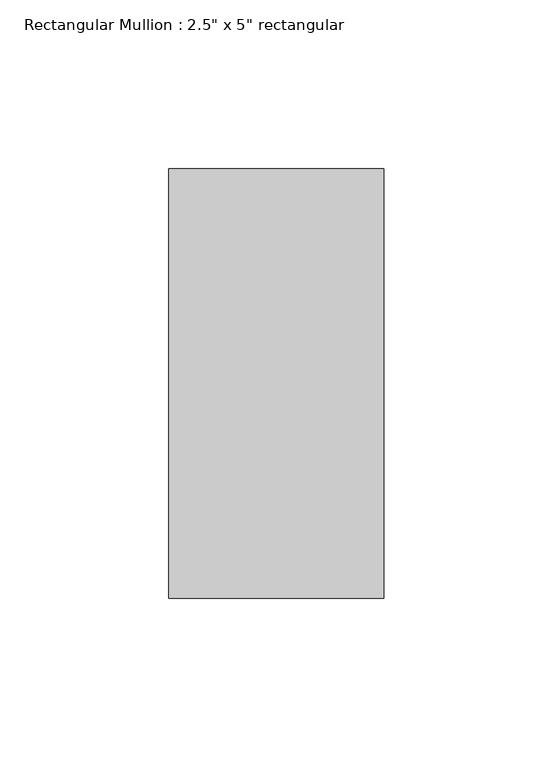
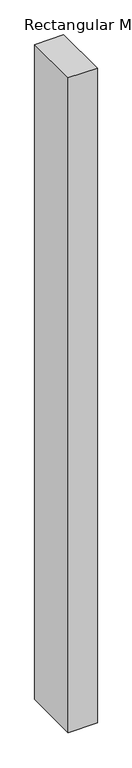
"""IFC4 building model written with IfcOpenShell, lengths in millimetres: member geometry."""

from ifc_helpers import new_model, si_unit, frame, origin, place, context, project, spatial, polyline, outline, extrude, source, transform, mapped, element, save


def member_e45318c1(model_context):
    return source(origin(), model_context, "Body", "SweptSolid", [
        extrude(outline(polyline([(31.75, 63.5), (31.75, -63.5), (-31.75, -63.5), (-31.75, 63.5), (31.75, 63.5)])), frame((0.0, 0.0, -1512.8617517), z_axis=(0.0, 0.0, 1.0), x_axis=(1.0, 0.0, 0.0)), (0.0, 0.0, 1.0), 1512.8617517),
    ])


if __name__ == "__main__":
    model = new_model("IFC4")
    model_context = context("Model", 3, world=origin())
    ifc_project = project(units=[si_unit("LENGTHUNIT", "METRE", prefix="MILLI")], contexts=[model_context])
    site = spatial("IfcSite", under=ifc_project)
    building = spatial("IfcBuilding", under=site)
    placement = place(None, origin())
    member_shape = member_e45318c1(model_context)
    element("IfcMember", 1, ObjectType="Rectangular Mullion : 2.5\" x 5\" rectangular", at=placement, inside=building, context=model_context, shape_type="MappedRepresentation", body=[
        mapped(member_shape, transform((0.0, 0.0, 0.0), x_axis=(1.0, 0.0, 0.0), y_axis=(0.0, 1.0, 0.0), z_axis=(0.0, 0.0, 1.0))),
    ])
    save(model, "model.ifc")

# Revit data of these elements
# Type "Rectangular Mullion : 2.5\" x 5\" rectangular"
#   built-in parameter 1007304 = 0.416667 (stored number, unit not read)
#   built-in parameter 1007301 = 0.104167 (stored number, unit not read)
#   built-in parameter 1007300 = 0.104167 (stored number, unit not read)
# Element 1 (IfcMember, "Rectangular Mullion : 2.5\" x 5\" rectangular")
#   Materials on its faces: "Aluminum"
# Materials
#   "Aluminum": class "Metal", colour RGB 247 247 247, transparency 0, Description = "Aluminum 6061", Cost = 0
